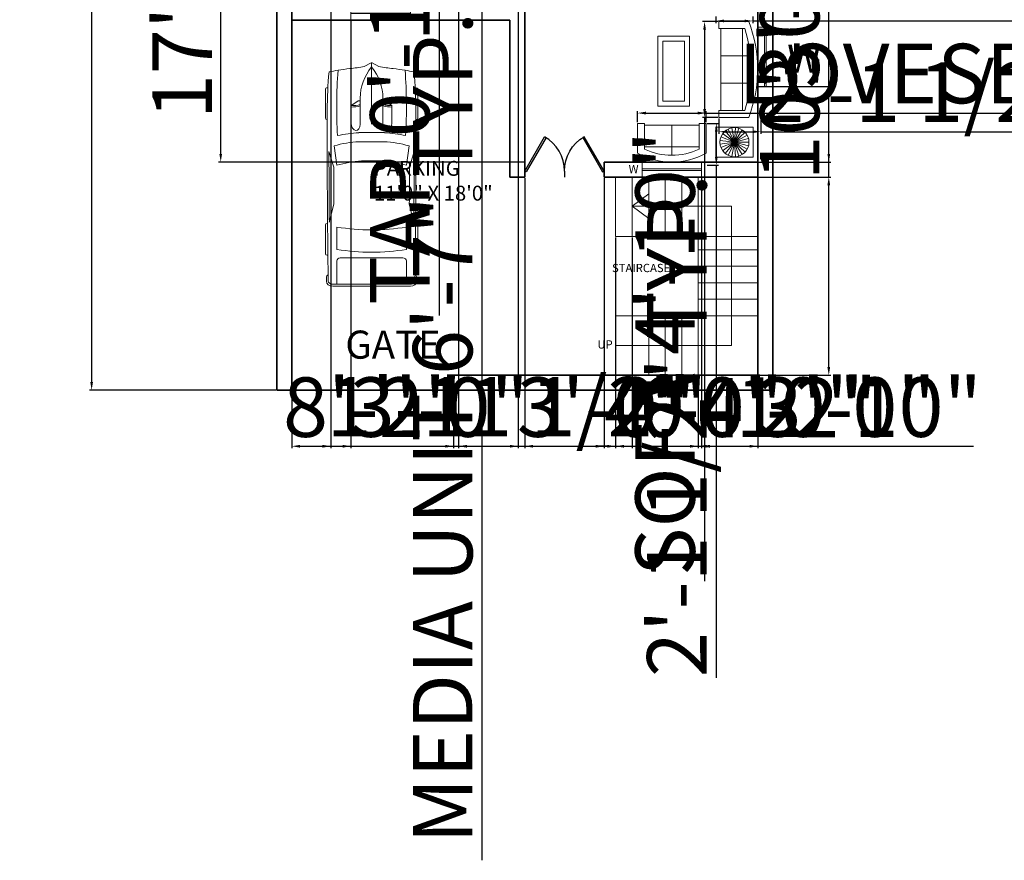
# Model space of a CAD drawing. Units: inches. Extents: x 2901 to 21549, y 2042 to 3828.
# Tile 1 of 10: x 3178 to 3774, y 2590 to 3099. Entities that reach past the tile are written whole.
import ezdxf

# ---------------------------------------------------------------- set-up
doc = ezdxf.new("R2010")
doc.units = ezdxf.units.IN
doc.layers.get('Defpoints').update_dxf_attribs({"color": 1})
for name, color, linetype, lineweight in [('A-ANNO-DIMS', 2, 'Continuous', 18), ('A-ANNO-TEXT', 7, 'Continuous', 18), ('A-AREA-IDEN', 7, 'Continuous', 18), ('A-DOOR', 3, 'Continuous', 25), ('A-FLOR-STRS', 7, 'Continuous', 20), ('A-FURN', 8, 'Continuous', 18), ('A-GLAZ', 4, 'Continuous', 18), ('A-SITE-PARK', 8, 'Continuous', 18), ('A-WALL', 7, 'Continuous', 35)]:
    doc.layers.add(name, color=color, linetype=linetype, lineweight=lineweight)
doc.styles.get("Standard").update_dxf_attribs({"font": 'arial.ttf'})
doc.dimstyles.new('ISO-25', dxfattribs={"dimtxt": 36, "dimasz": 5, "dimexe": 1.25, "dimexo": 0.625, "dimtad": 1, "dimdec": 0, "dimlunit": 3, "dimtxsty": 'Standard', "dimcen": 2.5, "dimadec": 0, "dimazin": 0, "dimtfac": 1, "dimtdec": 0, "dimtmove": 0, "dimatfit": 3, "dimfxl": 1, "dimarcsym": 0})

# ---------------------------------------------------------------- blocks, each defined once
blk = doc.blocks.new('*U23')
for p, q in [((0, 0), (0, -6)), ((40, 0), (40, -6))]:
    blk.add_line(p, q)
blk.add_lwpolyline([(0, 0), (20, 34.64), (21.52, 33.77), (1.52, -0.88)], close=True)
blk.add_arc((0, 0), 40, 0, 60)
blk = doc.blocks.new('Sofa - Roundback 7 ft.')
for p, q in [((-12.00002, -32.4421), (-12.00003, -6.5971)), ((11.99997, -32.4421), (11.99998, -6.5971)), ((-36.000027, -34), (-36.000027, -11.4696)), ((-35.999844, -13.3819), (35.9998, -13.3819)), ((35.99998, -34), (35.99998, -11.4696)), ((-36.000027, -32.4421), (35.99998, -32.4421))]:
    blk.add_line(p, q)
for points in [[(-36.000027, -34), (-42.000027, -34), (-42.000027, -8)], [(41.99998, -8), (41.99998, -34), (35.99998, -34)]]:
    blk.add_lwpolyline(points)
for centre, radius, start, end in [((0, -114.25), 114.25, 68.43141, 111.5686), ((-0.00001, -127.1968), 121.1968, 72.72033, 107.2797)]:
    blk.add_arc(centre, radius, start, end)
blk = doc.blocks.new('Sofa - Roundback Loveseat 5 ft.')
for p, q in [((0, -32.44198), (0, -5.99998)), ((-24, -33.99998), (-24, -11.46958)), ((-23.9998, -13.38178), (23.99986, -13.38178)), ((24.00004, -33.99998), (24.00004, -11.46958)), ((-24, -32.44198), (24.00004, -32.44198))]:
    blk.add_line(p, q)
for points in [[(-24, -33.99998), (-30, -33.99998), (-30, -7.99998)], [(30.00004, -7.99998), (30.00004, -33.99998), (24.00004, -33.99998)]]:
    blk.add_lwpolyline(points)
for centre, radius, start, end in [((0, -60.24998), 60.24998, 60.13715, 119.8628), ((0, -61.38438), 55.38444, 64.32083, 115.6792)]:
    blk.add_arc(centre, radius, start, end)
blk = doc.blocks.new('*U29')
for p, q in [((536, 950), (536, 936)), ((1182, 988), (568, 988)), ((1214, 950), (1214, 950)), ((2235, 810), (1899, 912)), ((3412, 904), (3030, 807)), ((3440, 942), (3440, 950)), ((3472, 988), (4087, 988)), ((4119, 950), (4119, 934)), ((4736, -851), (4736, 851)), ((1779, 801), (2195, 746)), ((3516, 746), (3994, 746)), ((4179, 670), (4179, -670)), ((4736, 746), (4242, 746)), ((4785, -832), (4785, 832)), ((820, 295), (918, 436)), ((918, 436), (1294, 436)), ((756, 241), (1313, 241)), ((816, 241), (816, 283)), ((1496, -274), (1496, 274)), ((1690, -267), (1690, 267)), ((2102, 216), (2102, -216)), ((4736, -267), (4736, 267)), ((83, 156), (3, 10)), ((0, 0), (1313, 0)), ((3, -10), (83, -156)), ((756, -241), (1313, -241)), ((816, -241), (816, -283)), ((820, -295), (918, -436)), ((918, -436), (1294, -436)), ((2195, -746), (1779, -801)), ((2235, -810), (1899, -912)), ((3412, -904), (3030, -807)), ((3994, -746), (3516, -746)), ((4242, -746), (4736, -746)), ((536, -950), (536, -936)), ((1182, -988), (568, -988)), ((1214, -950), (1214, -950)), ((3440, -942), (3440, -950)), ((3472, -988), (4087, -988)), ((4119, -950), (4119, -934))]:
    blk.add_line(p, q)
for centre, major_axis, ratio, start_param, end_param in [((6757, -699), (0, 7958), 0.842304, 1.367076, 1.39176), ((1046, -12468), (0, 13417), 0.842304, 0.00281, 0.075598), ((568, 950), (0, -37.6), 0.842304, 3.141593, 4.712389), ((1638, -268113), (0, 269063), 0.842304, -0.013397, 0.002797), ((1182, 950), (0, 37.6), 0.842304, -1.570796, 0), ((1638, -268113), (0, -269025), 0.842304, 3.133765, 3.140441), ((3472, 950), (0, -37.6), 0.842304, 3.141593, 4.712389), ((4087, 950), (0, 37.6), 0.842304, -1.570796, 0), ((4588, 910), (0, 56.4), 0.842304, -0.013017, 1.249894), ((1638, -268131), (0, 269121), 0.842304, -0.013397, -0.013017), ((4673, 851), (0, -75.2), 0.842304, 1.570796, 3.128196), ((4673, 832), (0, -133), 0.842304, 1.570796, 3.128196), ((6583, -699), (0, -7755), 0.842304, 4.528606, 4.561838), ((952, -15087), (0, -15833), 0.842304, 3.096046, 3.200911), ((3414, 137), (0, -2280), 0.842304, 4.449482, 4.652344), ((3436, 137), (0, 2077), 0.842304, 1.245306, 1.50788), ((3800, 71), (0, -2021), 0.842304, 4.372215, 4.640744), ((2433, -93125), (0, -93935), 0.842304, 3.134049, 3.144098), ((434, 0), (0, 3734), 0.842304, 4.511394, 4.913384), ((912, 0), (0, 3734), 0.842304, 4.511394, 4.913384), ((4242, 670), (0, 75.2), 0.842304, 0, 1.570796), ((-5194, 1331), (0, -6374), 0.842304, 1.385369, 1.434372), ((331, 432), (0, 696), 0.842304, 4.435146, 4.718221), ((361, 432), (0, 696), 0.842304, 4.435146, 4.718221), ((1290, 339), (161, -9), 0.603834, -1.395552, 1.581315), ((756, -1185), (0, 1427), 0.842304, 0, 0.590319), ((832, 283), (0, 18.8), 0.842304, 0.879714, 1.570796), ((16, 0), (0, -18.8), 0.842304, 4.131459, 5.293319), ((-5194, -1331), (0, 6374), 0.842304, -1.434372, -1.385369), ((756, 1185), (0, 1427), 0.842304, 2.551274, 3.141593), ((832, -283), (0, -18.8), 0.842304, 4.712389, 5.403472), ((331, -432), (0, -696), 0.842304, 1.564964, 1.848039), ((361, -432), (0, -696), 0.842304, 1.564964, 1.848039), ((3414, -137), (0, -2280), 0.842304, -1.510751, -1.307889), ((3436, -137), (0, -2077), 0.842304, -1.50788, -1.245306), ((3800, -71), (0, -2021), 0.842304, -1.499151, -1.230623), ((6583, 699), (0, 7755), 0.842304, 1.721348, 1.754579), ((6757, 699), (0, 7958), 0.842304, 1.749832, 1.774517), ((952, 15087), (0, -15833), 0.842304, -0.059319, 0.045547), ((2433, 93125), (0, -93935), 0.842304, -0.002505, 0.007544), ((4242, -670), (0, -75.2), 0.842304, 4.712389, 6.283185), ((4673, -832), (0, -133), 0.842304, 0.013397, 1.570796), ((1046, 12468), (0, -13417), 0.842304, -0.075598, -0.00281), ((568, -950), (0, 37.6), 0.842304, 1.570796, 3.141593), ((1638, 268113), (0, 269063), 0.842304, 3.138796, 3.15499), ((1182, -950), (0, -37.6), 0.842304, 0, 1.570796), ((1638, 268113), (0, -269025), 0.842304, 0.001152, 0.007828), ((3472, -950), (0, -37.6), 0.842304, -1.570796, 0), ((4087, -950), (0, 37.6), 0.842304, 3.141593, 4.712389), ((4588, -910), (0, -56.4), 0.842304, -1.249894, 0.013017), ((1638, 268131), (0, 269121), 0.842304, 3.15461, 3.15499), ((4673, -851), (0, 75.2), 0.842304, 3.15499, 4.712389)]:
    blk.add_ellipse(centre, major_axis=major_axis, ratio=ratio, start_param=start_param, end_param=end_param)
at = {"extrusion": (0, 0, -1)}
blk.add_ellipse((1290, -339), major_axis=(161, 9), ratio=0.603834, start_param=-1.395552, end_param=1.581315, dxfattribs=at)
blk = doc.blocks.new('*D31')
at = {"layer": 'A-ANNO-DIMS', "color": 0, "lineweight": -2, "transparency": 16777216}
for p, q in [((3333.44, 3474.48), (3220.78, 3474.48)), ((3222.03, 3469.48), (3222.03, 2879.48)), ((3333.44, 2874.48), (3220.78, 2874.48))]:
    blk.add_line(p, q, dxfattribs=at)
at = {"layer": 'A-ANNO-DIMS', "color": 0, "transparency": 16777216}
for points in [[(3221.19, 3469.48), (3222.86, 3469.48), (3222.03, 3474.48)], [(3221.19, 2879.48), (3222.86, 2879.48), (3222.03, 2874.48)]]:
    blk.add_solid(points, dxfattribs=at)
at = {"layer": 'Defpoints', "color": 0, "transparency": 16777216}
for p in [(3334.07, 3474.48), (3222.03, 2874.48), (3334.07, 2874.48)]:
    blk.add_point(p, dxfattribs=at)
at = {"layer": 'A-ANNO-DIMS', "color": 0, "transparency": 16777216, "insert": (3203.02, 3174.48), "char_height": 36, "attachment_point": 5, "rotation": 90}
blk.add_mtext("50'", dxfattribs=at)
blk = doc.blocks.new('WIN-36IN-9IN-WALL')
for p, q in [((0, 36), (9, 36)), ((0, 0), (0, 36)), ((4, 0), (4, 36)), ((5, 36), (5, 0)), ((9, 36), (9, 0)), ((9, 0), (0, 0))]:
    blk.add_line(p, q)
blk = doc.blocks.new('*U24')
blk.add_line((-4.41, 0), (4.41, 0))
blk = doc.blocks.new('*U25')
at = {"color": 0, "linetype": 'ByBlock', "lineweight": -2, "transparency": 16777216}
for p, rotation in [((3609.05, 3028.55), 115.1999999999997), ((3610.1, 3028.89), 100.7999999999996), ((3611.21, 3028.96), 86.39999999999972), ((3612.29, 3028.76), 71.99999999999977), ((3606.83, 3026.19), 158.3999999999996), ((3607.36, 3027.15), 143.9999999999996), ((3608.12, 3027.96), 129.5999999999996), ((3613.29, 3028.29), 57.59999999999982), ((3614.14, 3027.58), 43.19999999999986), ((3614.79, 3026.69), 28.7999999999999), ((3615.2, 3025.66), 14.39999999999998), ((3606.56, 3025.12), 172.7999999999996), ((3606.56, 3024.01), 187.1999999999994), ((3606.83, 3022.94), 201.5999999999995), ((3607.36, 3021.97), 215.9999999999995), ((3608.12, 3021.17), 230.3999999999995), ((3609.05, 3020.58), 244.7999999999995), ((3610.1, 3020.23), 259.1999999999994), ((3611.21, 3020.17), 273.5999999999994), ((3612.29, 3020.37), 287.9999999999993), ((3613.29, 3020.84), 302.3999999999992), ((3614.14, 3021.55), 316.7999999999993), ((3614.79, 3022.44), 331.1999999999992), ((3615.2, 3023.47), 345.5999999999992)]:
    blk.add_blockref('*U24', p, dxfattribs=dict(at, rotation=rotation))
blk.add_blockref('*U24', (3615.34, 3024.56), dxfattribs=at)
blk = doc.blocks.new('TABLE-END-DECOR')
blk.add_lwpolyline([(0, 18.24), (22.47, 18.24), (22.47, 0), (0, 0)], close=True)
blk.add_circle((11.23, 9.12), 8.81)
blk.add_blockref('*U25', (-3599.7, -3015.44))
blk = doc.blocks.new('*D44')
at = {"layer": 'A-ANNO-DIMS', "color": 0, "lineweight": -2, "transparency": 16777216}
for p, q in [((3432.19, 3305.97), (3432.19, 3310.97)), ((3431.32, 3300.97), (3433.44, 3300.97)), ((3432.19, 3300.97), (3432.19, 3290.97)), ((3431.32, 3290.97), (3433.44, 3290.97)), ((3432.19, 3285.97), (3432.19, 2919.63))]:
    blk.add_line(p, q, dxfattribs=at)
at = {"layer": 'A-ANNO-DIMS', "color": 0, "transparency": 16777216}
for points in [[(3431.36, 3305.97), (3433.02, 3305.97), (3432.19, 3300.97)], [(3431.36, 3285.97), (3433.02, 3285.97), (3432.19, 3290.97)]]:
    blk.add_solid(points, dxfattribs=at)
at = {"layer": 'Defpoints', "color": 0, "transparency": 16777216}
for p in [(3430.69, 3300.97), (3430.69, 3290.97), (3432.19, 3290.97)]:
    blk.add_point(p, dxfattribs=at)
at = {"layer": 'A-ANNO-DIMS', "color": 0, "transparency": 16777216, "insert": (3413.18, 3100.3), "char_height": 36, "attachment_point": 5, "rotation": 90}
blk.add_mtext('TAP 0\'-10" TYP.', dxfattribs=at)
blk = doc.blocks.new('*D48')
at = {"layer": 'A-ANNO-DIMS', "color": 0, "lineweight": -2, "transparency": 16777216}
for p, q in [((3552.33, 3036.58), (3552.33, 3043.43)), ((3557.33, 3042.18), (3588.77, 3042.18)), ((3593.77, 3036.58), (3593.77, 3043.43)), ((3593.77, 3042.18), (4181.25, 3042.18))]:
    blk.add_line(p, q, dxfattribs=at)
at = {"layer": 'A-ANNO-DIMS', "color": 0, "transparency": 16777216}
for points in [[(3557.33, 3043.01), (3557.33, 3041.34), (3552.33, 3042.18)], [(3588.77, 3043.01), (3588.77, 3041.34), (3593.77, 3042.18)]]:
    blk.add_solid(points, dxfattribs=at)
at = {"layer": 'Defpoints', "color": 0, "transparency": 16777216}
for p in [(3593.77, 3042.18), (3552.33, 3035.96), (3593.77, 3035.96)]:
    blk.add_point(p, dxfattribs=at)
at = {"layer": 'A-ANNO-DIMS', "color": 0, "transparency": 16777216, "insert": (3890.01, 3061.44), "char_height": 36, "attachment_point": 5}
blk.add_mtext('LOVESEAT 3\'-5 1/2" TYP.', dxfattribs=at)
blk = doc.blocks.new('*D49')
at = {"layer": 'A-ANNO-DIMS', "color": 0, "lineweight": -2, "transparency": 16777216}
for p, q in [((3594.39, 3035.96), (3601.23, 3035.96)), ((3599.98, 3030.96), (3599.98, 3015.64)), ((3594.39, 3010.64), (3601.23, 3010.64)), ((3599.98, 3010.64), (3599.98, 2700.45))]:
    blk.add_line(p, q, dxfattribs=at)
at = {"layer": 'A-ANNO-DIMS', "color": 0, "transparency": 16777216}
for points in [[(3599.15, 3030.96), (3600.81, 3030.96), (3599.98, 3035.96)], [(3599.15, 3015.64), (3600.81, 3015.64), (3599.98, 3010.64)]]:
    blk.add_solid(points, dxfattribs=at)
at = {"layer": 'Defpoints', "color": 0, "transparency": 16777216}
for p in [(3593.77, 3035.96), (3593.77, 3010.64), (3599.98, 3010.64)]:
    blk.add_point(p, dxfattribs=at)
at = {"layer": 'A-ANNO-DIMS', "color": 0, "transparency": 16777216, "insert": (3580.74, 2853.04), "char_height": 36, "attachment_point": 5, "rotation": 90}
blk.add_mtext('2\'-1 1/2" TYP.', dxfattribs=at)
blk = doc.blocks.new('*D50')
at = {"layer": 'A-ANNO-DIMS', "color": 0, "lineweight": -2, "transparency": 16777216}
for p, q in [((3599.61, 3100.68), (3599.61, 3096.69)), ((3604.61, 3097.94), (3617.08, 3097.94)), ((3622.08, 3100.68), (3622.08, 3096.69)), ((3622.08, 3097.94), (4251.18, 3097.94))]:
    blk.add_line(p, q, dxfattribs=at)
at = {"layer": 'A-ANNO-DIMS', "color": 0, "transparency": 16777216}
for points in [[(3604.61, 3098.77), (3604.61, 3097.1), (3599.61, 3097.94)], [(3617.08, 3098.77), (3617.08, 3097.1), (3622.08, 3097.94)]]:
    blk.add_solid(points, dxfattribs=at)
at = {"layer": 'Defpoints', "color": 0, "transparency": 16777216}
for p in [(3599.61, 3101.31), (3622.08, 3101.31), (3622.08, 3097.94)]:
    blk.add_point(p, dxfattribs=at)
at = {"layer": 'A-ANNO-DIMS', "color": 0, "transparency": 16777216, "insert": (3939.13, 3117.18), "char_height": 36, "attachment_point": 5}
blk.add_mtext('END TABLE 1\'-10 1/2" TYP.', dxfattribs=at)
blk = doc.blocks.new('*D52')
at = {"layer": 'A-ANNO-DIMS', "color": 0, "lineweight": -2, "transparency": 16777216}
for p, q in [((3469.26, 3197.35), (3456.81, 3197.35)), ((3458.06, 3192.35), (3458.06, 3123.52)), ((3469.26, 3118.52), (3456.81, 3118.52)), ((3458.06, 3118.52), (3458.06, 2589.92))]:
    blk.add_line(p, q, dxfattribs=at)
at = {"layer": 'A-ANNO-DIMS', "color": 0, "transparency": 16777216}
for points in [[(3457.23, 3192.35), (3458.9, 3192.35), (3458.06, 3197.35)], [(3457.23, 3123.52), (3458.9, 3123.52), (3458.06, 3118.52)]]:
    blk.add_solid(points, dxfattribs=at)
at = {"layer": 'Defpoints', "color": 0, "transparency": 16777216}
for p in [(3469.89, 3197.35), (3458.06, 3118.52), (3469.89, 3118.52)]:
    blk.add_point(p, dxfattribs=at)
at = {"layer": 'A-ANNO-DIMS', "color": 0, "transparency": 16777216, "insert": (3439.06, 2851.72), "char_height": 36, "attachment_point": 5, "rotation": 90}
blk.add_mtext('MEDIA UNIT 6\'-7" TYP.', dxfattribs=at)
blk = doc.blocks.new('*D54')
at = {"layer": 'A-ANNO-DIMS', "color": 0, "lineweight": -2, "transparency": 16777216}
for p, q in [((3536.12, 3164.87), (3536.12, 3153.97)), ((3604.61, 3164.87), (3604.61, 3153.97)), ((3541.12, 3155.22), (3599.61, 3155.22)), ((3604.61, 3155.22), (4090.43, 3155.22))]:
    blk.add_line(p, q, dxfattribs=at)
at = {"layer": 'A-ANNO-DIMS', "color": 0, "transparency": 16777216}
for points in [[(3541.12, 3156.05), (3541.12, 3154.38), (3536.12, 3155.22)], [(3599.61, 3156.05), (3599.61, 3154.38), (3604.61, 3155.22)]]:
    blk.add_solid(points, dxfattribs=at)
at = {"layer": 'Defpoints', "color": 0, "transparency": 16777216}
for p in [(3536.12, 3165.49), (3604.61, 3165.49), (3604.61, 3155.22)]:
    blk.add_point(p, dxfattribs=at)
at = {"layer": 'A-ANNO-DIMS', "color": 0, "transparency": 16777216, "insert": (3850.02, 3174.46), "char_height": 36, "attachment_point": 5}
blk.add_mtext('DINING SET 5\'-8 1/2"', dxfattribs=at)
blk = doc.blocks.new('*D56')
at = {"layer": 'A-ANNO-DIMS', "color": 0, "lineweight": -2, "transparency": 16777216}
for p, q in [((3600.96, 3097.61), (3591.63, 3097.61)), ((3592.88, 3092.61), (3592.88, 3044.6)), ((3600.96, 3039.6), (3591.63, 3039.6)), ((3592.88, 3039.6), (3592.88, 2758.95))]:
    blk.add_line(p, q, dxfattribs=at)
at = {"layer": 'A-ANNO-DIMS', "color": 0, "transparency": 16777216}
for points in [[(3592.05, 3092.61), (3593.72, 3092.61), (3592.88, 3097.61)], [(3592.05, 3044.6), (3593.72, 3044.6), (3592.88, 3039.6)]]:
    blk.add_solid(points, dxfattribs=at)
at = {"layer": 'Defpoints', "color": 0, "transparency": 16777216}
for p in [(3601.59, 3097.61), (3592.88, 3039.6), (3601.59, 3039.6)]:
    blk.add_point(p, dxfattribs=at)
at = {"layer": 'A-ANNO-DIMS', "color": 0, "transparency": 16777216, "insert": (3573.63, 2896.77), "char_height": 36, "attachment_point": 5, "rotation": 90}
blk.add_mtext('SOFA 4\'-10"', dxfattribs=at)
blk = doc.blocks.new('*D57')
at = {"layer": 'A-ANNO-DIMS', "color": 0, "lineweight": -2, "transparency": 16777216}
for p, q in [((3601.59, 3038.97), (3601.59, 3029.64)), ((3626.91, 3038.97), (3626.91, 3029.64)), ((3606.59, 3030.89), (3621.91, 3030.89)), ((3626.91, 3030.89), (3813.36, 3030.89))]:
    blk.add_line(p, q, dxfattribs=at)
at = {"layer": 'A-ANNO-DIMS', "color": 0, "transparency": 16777216}
for points in [[(3606.59, 3031.73), (3606.59, 3030.06), (3601.59, 3030.89)], [(3621.91, 3031.73), (3621.91, 3030.06), (3626.91, 3030.89)]]:
    blk.add_solid(points, dxfattribs=at)
at = {"layer": 'Defpoints', "color": 0, "transparency": 16777216}
for p in [(3601.59, 3039.6), (3626.91, 3039.6), (3626.91, 3030.89)]:
    blk.add_point(p, dxfattribs=at)
at = {"layer": 'A-ANNO-DIMS', "color": 0, "transparency": 16777216, "insert": (3722.63, 3050.13), "char_height": 36, "attachment_point": 5}
blk.add_mtext('2\'-1 1/2"', dxfattribs=at)
blk = doc.blocks.new('*D62')
at = {"layer": 'A-ANNO-DIMS', "color": 0, "lineweight": -2, "transparency": 16777216}
for p, q in [((3343.07, 2873.85), (3343.07, 2839.28)), ((3441, 2873.85), (3441, 2839.28)), ((3348.07, 2840.53), (3436, 2840.53))]:
    blk.add_line(p, q, dxfattribs=at)
at = {"layer": 'A-ANNO-DIMS', "color": 0, "transparency": 16777216}
for points in [[(3348.07, 2841.36), (3348.07, 2839.69), (3343.07, 2840.53)], [(3436, 2841.36), (3436, 2839.69), (3441, 2840.53)]]:
    blk.add_solid(points, dxfattribs=at)
at = {"layer": 'Defpoints', "color": 0, "transparency": 16777216}
for p in [(3343.07, 2874.48), (3441, 2874.48), (3441, 2840.53)]:
    blk.add_point(p, dxfattribs=at)
at = {"layer": 'A-ANNO-DIMS', "color": 0, "transparency": 16777216, "insert": (3392.04, 2859.53), "char_height": 36, "attachment_point": 5}
blk.add_mtext('8\'-2"', dxfattribs=at)
blk = doc.blocks.new('*D63')
at = {"layer": 'A-ANNO-DIMS', "color": 0, "lineweight": -2, "transparency": 16777216}
for p, q in [((3539.07, 2882.85), (3539.07, 2839.28)), ((3589.07, 2882.85), (3589.07, 2839.28)), ((3544.07, 2840.53), (3584.07, 2840.53)), ((3589.07, 2840.53), (3692.47, 2840.53))]:
    blk.add_line(p, q, dxfattribs=at)
at = {"layer": 'A-ANNO-DIMS', "color": 0, "transparency": 16777216}
for points in [[(3544.07, 2841.36), (3544.07, 2839.69), (3539.07, 2840.53)], [(3584.07, 2841.36), (3584.07, 2839.69), (3589.07, 2840.53)]]:
    blk.add_solid(points, dxfattribs=at)
at = {"layer": 'Defpoints', "color": 0, "transparency": 16777216}
for p in [(3539.07, 2883.48), (3589.07, 2883.48), (3589.07, 2840.53)]:
    blk.add_point(p, dxfattribs=at)
at = {"layer": 'A-ANNO-DIMS', "color": 0, "transparency": 16777216, "insert": (3643.27, 2859.23), "char_height": 36, "attachment_point": 5}
blk.add_mtext('4\'-2"', dxfattribs=at)
blk = doc.blocks.new('*D64')
at = {"layer": 'A-ANNO-DIMS', "color": 0, "lineweight": -2, "transparency": 16777216}
for p, q in [((3589.07, 2882.85), (3589.07, 2839.28)), ((3625.07, 2882.85), (3625.07, 2839.28)), ((3594.07, 2840.53), (3620.07, 2840.53)), ((3625.07, 2840.53), (3726.99, 2840.53))]:
    blk.add_line(p, q, dxfattribs=at)
at = {"layer": 'A-ANNO-DIMS', "color": 0, "transparency": 16777216}
for points in [[(3594.07, 2841.36), (3594.07, 2839.69), (3589.07, 2840.53)], [(3620.07, 2841.36), (3620.07, 2839.69), (3625.07, 2840.53)]]:
    blk.add_solid(points, dxfattribs=at)
at = {"layer": 'Defpoints', "color": 0, "transparency": 16777216}
for p in [(3589.07, 2883.48), (3625.07, 2883.48), (3625.07, 2840.53)]:
    blk.add_point(p, dxfattribs=at)
at = {"layer": 'A-ANNO-DIMS', "color": 0, "transparency": 16777216, "insert": (3678.53, 2859.55), "char_height": 36, "attachment_point": 5}
blk.add_mtext('3\'-0"', dxfattribs=at)
blk = doc.blocks.new('*D65')
at = {"layer": 'A-ANNO-DIMS', "color": 0, "lineweight": -2, "transparency": 16777216}
for p, q in [((3668.02, 3003.48), (3668.02, 3130.01)), ((3625.69, 3003.48), (3669.27, 3003.48)), ((3668.02, 2888.48), (3668.02, 2998.48)), ((3625.69, 2883.48), (3669.27, 2883.48))]:
    blk.add_line(p, q, dxfattribs=at)
at = {"layer": 'A-ANNO-DIMS', "color": 0, "transparency": 16777216}
for points in [[(3667.19, 2998.48), (3668.85, 2998.48), (3668.02, 3003.48)], [(3667.19, 2888.48), (3668.85, 2888.48), (3668.02, 2883.48)]]:
    blk.add_solid(points, dxfattribs=at)
at = {"layer": 'Defpoints', "color": 0, "transparency": 16777216}
for p in [(3625.07, 3003.48), (3668.02, 3003.48), (3625.07, 2883.48)]:
    blk.add_point(p, dxfattribs=at)
at = {"layer": 'A-ANNO-DIMS', "color": 0, "transparency": 16777216, "insert": (3649.01, 3069.24), "char_height": 36, "attachment_point": 5, "rotation": 90}
blk.add_mtext('10\'-0"', dxfattribs=at)
blk = doc.blocks.new('*D66')
at = {"layer": 'A-ANNO-DIMS', "color": 0, "lineweight": -2, "transparency": 16777216}
for p, q in [((3484.07, 3002.85), (3484.07, 2839.28)), ((3532.07, 3002.85), (3532.07, 2839.28)), ((3489.07, 2840.53), (3527.07, 2840.53)), ((3532.07, 2840.53), (3635.47, 2840.53))]:
    blk.add_line(p, q, dxfattribs=at)
at = {"layer": 'A-ANNO-DIMS', "color": 0, "transparency": 16777216}
for points in [[(3489.07, 2841.36), (3489.07, 2839.69), (3484.07, 2840.53)], [(3527.07, 2841.36), (3527.07, 2839.69), (3532.07, 2840.53)]]:
    blk.add_solid(points, dxfattribs=at)
at = {"layer": 'Defpoints', "color": 0, "transparency": 16777216}
for p in [(3484.07, 3003.48), (3532.07, 3003.48), (3532.07, 2840.53)]:
    blk.add_point(p, dxfattribs=at)
at = {"layer": 'A-ANNO-DIMS', "color": 0, "transparency": 16777216, "insert": (3586.27, 2859.53), "char_height": 36, "attachment_point": 5}
blk.add_mtext('4\'-0"', dxfattribs=at)
blk = doc.blocks.new('*D67')
at = {"layer": 'A-ANNO-DIMS', "color": 0, "lineweight": -2, "transparency": 16777216}
for p, q in [((3484.07, 3013.1), (3484.07, 3509.68)), ((3625.07, 3228.1), (3625.07, 3509.68)), ((3489.07, 3508.43), (3620.07, 3508.43))]:
    blk.add_line(p, q, dxfattribs=at)
at = {"layer": 'A-ANNO-DIMS', "color": 0, "transparency": 16777216}
for points in [[(3489.07, 3509.26), (3489.07, 3507.59), (3484.07, 3508.43)], [(3620.07, 3509.26), (3620.07, 3507.59), (3625.07, 3508.43)]]:
    blk.add_solid(points, dxfattribs=at)
at = {"layer": 'Defpoints', "color": 0, "transparency": 16777216}
for p in [(3625.07, 3508.43), (3625.07, 3227.48), (3484.07, 3012.48)]:
    blk.add_point(p, dxfattribs=at)
at = {"layer": 'A-ANNO-DIMS', "color": 0, "transparency": 16777216, "insert": (3554.57, 3527.43), "char_height": 36, "attachment_point": 5}
blk.add_mtext('11\'-9"', dxfattribs=at)
blk = doc.blocks.new('*D68')
at = {"layer": 'A-ANNO-DIMS', "color": 0, "lineweight": -2, "transparency": 16777216}
for p, q in [((3531.44, 3227.48), (3298.87, 3227.48)), ((3300.12, 3017.48), (3300.12, 3222.48)), ((3483.44, 3012.48), (3298.87, 3012.48))]:
    blk.add_line(p, q, dxfattribs=at)
at = {"layer": 'A-ANNO-DIMS', "color": 0, "transparency": 16777216}
for points in [[(3299.29, 3222.48), (3300.95, 3222.48), (3300.12, 3227.48)], [(3299.29, 3017.48), (3300.95, 3017.48), (3300.12, 3012.48)]]:
    blk.add_solid(points, dxfattribs=at)
at = {"layer": 'Defpoints', "color": 0, "transparency": 16777216}
for p in [(3300.12, 3227.48), (3532.07, 3227.48), (3484.07, 3012.48)]:
    blk.add_point(p, dxfattribs=at)
at = {"layer": 'A-ANNO-DIMS', "color": 0, "transparency": 16777216, "insert": (3281.42, 3119.98), "char_height": 36, "attachment_point": 5, "rotation": 90}
blk.add_mtext('17\'-11"', dxfattribs=at)
blk = doc.blocks.new('*D73')
at = {"layer": 'A-ANNO-DIMS', "color": 0, "lineweight": -2, "transparency": 16777216}
for p, q in [((3668.02, 3058.19), (3668.02, 3244)), ((3625.69, 3058.19), (3669.27, 3058.19)), ((3668.02, 3017.48), (3668.02, 3053.19)), ((3625.69, 3012.48), (3669.27, 3012.48))]:
    blk.add_line(p, q, dxfattribs=at)
at = {"layer": 'A-ANNO-DIMS', "color": 0, "transparency": 16777216}
for points in [[(3667.19, 3053.19), (3668.85, 3053.19), (3668.02, 3058.19)], [(3667.19, 3017.48), (3668.85, 3017.48), (3668.02, 3012.48)]]:
    blk.add_solid(points, dxfattribs=at)
at = {"layer": 'Defpoints', "color": 0, "transparency": 16777216}
for p in [(3625.07, 3058.19), (3668.02, 3058.19), (3625.07, 3012.48)]:
    blk.add_point(p, dxfattribs=at)
at = {"layer": 'A-ANNO-DIMS', "color": 0, "transparency": 16777216, "insert": (3648.77, 3153.6), "char_height": 36, "attachment_point": 5, "rotation": 90}
blk.add_mtext('3\'-9 1/2"', dxfattribs=at)
blk = doc.blocks.new('*D75')
at = {"layer": 'A-ANNO-DIMS', "color": 0, "lineweight": -2, "transparency": 16777216}
for p, q in [((3343.07, 3097.85), (3343.07, 2839.28)), ((3378.91, 3097.85), (3378.91, 2839.28)), ((3348.07, 2840.53), (3373.91, 2840.53)), ((3378.91, 2840.53), (3480.83, 2840.53))]:
    blk.add_line(p, q, dxfattribs=at)
at = {"layer": 'A-ANNO-DIMS', "color": 0, "transparency": 16777216}
for points in [[(3348.07, 2841.36), (3348.07, 2839.69), (3343.07, 2840.53)], [(3373.91, 2841.36), (3373.91, 2839.69), (3378.91, 2840.53)]]:
    blk.add_solid(points, dxfattribs=at)
at = {"layer": 'Defpoints', "color": 0, "transparency": 16777216}
for p in [(3343.07, 3098.48), (3378.91, 3098.48), (3378.91, 2840.53)]:
    blk.add_point(p, dxfattribs=at)
at = {"layer": 'A-ANNO-DIMS', "color": 0, "transparency": 16777216, "insert": (3432.37, 2859.55), "char_height": 36, "attachment_point": 5}
blk.add_mtext('3\'-0"', dxfattribs=at)
blk = doc.blocks.new('*D76')
at = {"layer": 'A-ANNO-DIMS', "color": 0, "lineweight": -2, "transparency": 16777216}
for p, q in [((3591.05, 3002.85), (3591.05, 2839.28)), ((3625.07, 3002.85), (3625.07, 2839.28)), ((3596.05, 2840.53), (3620.07, 2840.53)), ((3625.07, 2840.53), (3755.6, 2840.53))]:
    blk.add_line(p, q, dxfattribs=at)
at = {"layer": 'A-ANNO-DIMS', "color": 0, "transparency": 16777216}
for points in [[(3596.05, 2841.36), (3596.05, 2839.69), (3591.05, 2840.53)], [(3620.07, 2841.36), (3620.07, 2839.69), (3625.07, 2840.53)]]:
    blk.add_solid(points, dxfattribs=at)
at = {"layer": 'Defpoints', "color": 0, "transparency": 16777216}
for p in [(3591.05, 3003.48), (3625.07, 3003.48), (3625.07, 2840.53)]:
    blk.add_point(p, dxfattribs=at)
at = {"layer": 'A-ANNO-DIMS', "color": 0, "transparency": 16777216, "insert": (3692.84, 2859.53), "char_height": 36, "attachment_point": 5}
blk.add_mtext('2\'-10"', dxfattribs=at)
blk = doc.blocks.new('*D78')
at = {"layer": 'A-ANNO-DIMS', "color": 0, "lineweight": -2, "transparency": 16777216}
for p, q in [((3343.07, 3230.85), (3343.07, 2839.28)), ((3366.66, 3230.85), (3366.66, 2839.28)), ((3348.07, 2840.53), (3361.66, 2840.53)), ((3366.66, 2840.53), (3577.07, 2840.53))]:
    blk.add_line(p, q, dxfattribs=at)
at = {"layer": 'A-ANNO-DIMS', "color": 0, "transparency": 16777216}
for points in [[(3348.07, 2841.36), (3348.07, 2839.69), (3343.07, 2840.53)], [(3361.66, 2841.36), (3361.66, 2839.69), (3366.66, 2840.53)]]:
    blk.add_solid(points, dxfattribs=at)
at = {"layer": 'Defpoints', "color": 0, "transparency": 16777216}
for p in [(3343.07, 3231.48), (3366.66, 3231.48), (3366.66, 2840.53)]:
    blk.add_point(p, dxfattribs=at)
at = {"layer": 'A-ANNO-DIMS', "color": 0, "transparency": 16777216, "insert": (3474.37, 2859.77), "char_height": 36, "attachment_point": 5}
blk.add_mtext('1\'-11 1/2"', dxfattribs=at)
blk = doc.blocks.new('*D84')
at = {"layer": 'A-ANNO-DIMS', "color": 0, "lineweight": -2, "transparency": 16777216}
for p, q in [((3444.07, 3230.85), (3444.07, 2839.28)), ((3480.07, 3230.85), (3480.07, 2839.28)), ((3449.07, 2840.53), (3475.07, 2840.53)), ((3480.07, 2840.53), (3581.99, 2840.53))]:
    blk.add_line(p, q, dxfattribs=at)
at = {"layer": 'A-ANNO-DIMS', "color": 0, "transparency": 16777216}
for points in [[(3449.07, 2841.36), (3449.07, 2839.69), (3444.07, 2840.53)], [(3475.07, 2841.36), (3475.07, 2839.69), (3480.07, 2840.53)]]:
    blk.add_solid(points, dxfattribs=at)
at = {"layer": 'Defpoints', "color": 0, "transparency": 16777216}
for p in [(3444.07, 3231.48), (3480.07, 3231.48), (3480.07, 2840.53)]:
    blk.add_point(p, dxfattribs=at)
at = {"layer": 'A-ANNO-DIMS', "color": 0, "transparency": 16777216, "insert": (3533.53, 2859.55), "char_height": 36, "attachment_point": 5}
blk.add_mtext('3\'-0"', dxfattribs=at)
blk = doc.blocks.new('*D85')
at = {"layer": 'A-ANNO-DIMS', "color": 0, "lineweight": -2, "transparency": 16777216}
for p, q in [((3539.07, 2966.85), (3539.07, 2839.28)), ((3549.07, 2966.85), (3549.07, 2839.28)), ((3534.07, 2840.53), (3529.07, 2840.53)), ((3539.07, 2840.53), (3549.07, 2840.53)), ((3554.07, 2840.53), (3683.99, 2840.53))]:
    blk.add_line(p, q, dxfattribs=at)
at = {"layer": 'A-ANNO-DIMS', "color": 0, "transparency": 16777216}
for points in [[(3534.07, 2841.36), (3534.07, 2839.69), (3539.07, 2840.53)], [(3554.07, 2841.36), (3554.07, 2839.69), (3549.07, 2840.53)]]:
    blk.add_solid(points, dxfattribs=at)
at = {"layer": 'Defpoints', "color": 0, "transparency": 16777216}
for p in [(3539.07, 2967.48), (3549.07, 2967.48), (3549.07, 2840.53)]:
    blk.add_point(p, dxfattribs=at)
at = {"layer": 'A-ANNO-DIMS', "color": 0, "transparency": 16777216, "insert": (3621.53, 2859.53), "char_height": 36, "attachment_point": 5}
blk.add_mtext('0\'-10"', dxfattribs=at)

msp = doc.modelspace()

# ---------------------------------------------------------------- linework, layer by layer
at = {"layer": 'A-FLOR-STRS'}
for p, q in [((3539.07, 2967.48), (3539.07, 3003.48)), ((3549.07, 2967.48), (3549.07, 3003.48)), ((3559.07, 2967.48), (3559.07, 3003.48)), ((3569.07, 2967.48), (3569.07, 3003.48)), ((3579.07, 2967.48), (3579.07, 3003.48)), ((3589.07, 3003.48), (3589.07, 2967.48)), ((3589.07, 2967.48), (3589.07, 3003.48)), ((3549.07, 2985.89), (3559.07, 2993.4)), ((3609.23, 2985.89), (3549.07, 2985.89)), ((3549.07, 2985.89), (3559.07, 2978.37)), ((3609.23, 2901.48), (3609.23, 2985.89)), ((3625.07, 2967.48), (3539.07, 2967.48)), ((3589.07, 2919.48), (3589.07, 2967.48)), ((3589.07, 2959.48), (3625.07, 2959.48)), ((3589.07, 2949.48), (3625.07, 2949.48)), ((3589.07, 2939.48), (3625.07, 2939.48)), ((3589.07, 2929.48), (3625.07, 2929.48)), ((3625.07, 2919.48), (3539.07, 2919.48)), ((3539.07, 2919.48), (3539.07, 2883.48)), ((3549.07, 2919.48), (3549.07, 2883.48)), ((3559.07, 2919.48), (3559.07, 2883.48)), ((3569.07, 2919.48), (3569.07, 2883.48)), ((3579.07, 2919.48), (3579.07, 2883.48)), ((3589.07, 2919.48), (3589.07, 2883.48)), ((3589.07, 2919.48), (3625.07, 2919.48)), ((3539.07, 2901.48), (3609.23, 2901.48))]:
    msp.add_line(p, q, dxfattribs=at)
at = {"layer": 'A-FURN'}
for points in [[(3564.66, 3088.7), (3583.75, 3088.7), (3583.75, 3046.38), (3564.66, 3046.38)], [(3567.66, 3085.7), (3580.75, 3085.7), (3580.75, 3049.38), (3567.66, 3049.38)]]:
    msp.add_lwpolyline(points, close=True, dxfattribs=at)
at = {"layer": 'A-WALL'}
for p, q in [((3343.07, 2883.48), (3343.07, 3465.48)), ((3625.07, 3465.48), (3625.07, 2883.48)), ((3484.07, 3012.48), (3484.07, 3231.48)), ((3343.07, 3098.48), (3475.07, 3098.48)), ((3475.07, 3003.48), (3475.07, 3098.48)), ((3484.07, 3012.48), (3484.07, 3003.48)), ((3625.07, 3012.48), (3532.07, 3012.48)), ((3532.07, 3012.48), (3532.07, 3003.48)), ((3484.07, 3003.48), (3475.07, 3003.48)), ((3625.07, 3003.48), (3532.07, 3003.48)), ((3343.07, 2883.48), (3343.07, 2874.48)), ((3625.07, 2883.48), (3441, 2883.48)), ((3441, 2874.48), (3441, 2883.48))]:
    msp.add_line(p, q, dxfattribs=at)
msp.add_lwpolyline([(3634.07, 3474.48), (3634.07, 2874.48), (3334.07, 2874.48), (3334.07, 3474.48)], close=True, dxfattribs=at)

# ---------------------------------------------------------------- block references
at = {"layer": 'A-DOOR', "yscale": 0.6000000000000111, "zscale": 0.6000000000000111}
for p, xscale in [((3484.07, 3007.08), 0.6000000000000111), ((3532.07, 3007.08), -0.6000000000000111)]:
    msp.add_blockref('*U23', p, dxfattribs=dict(at, xscale=xscale))
at = {"layer": 'A-FURN', "yscale": 0.690663340395338, "zscale": 0.690663340395338}
for name, p, xscale, rotation in [('Sofa - Roundback 7 ft.', (3625.07, 3068.6), 0.690663340395338, 270), ('Sofa - Roundback Loveseat 5 ft.', (3573.05, 3012.48), -0.690663340395338, 180)]:
    msp.add_blockref(name, p, dxfattribs=dict(at, xscale=xscale, rotation=rotation))
at = {"layer": 'A-FURN'}
msp.add_blockref('TABLE-END-DECOR', (3599.7, 3015.44), dxfattribs=at)
at = {"layer": 'A-GLAZ', "rotation": 270}
for p in [(3378.91, 3107.48), (3555.05, 3012.48)]:
    msp.add_blockref('WIN-36IN-9IN-WALL', p, dxfattribs=at)
at = {"layer": 'A-GLAZ'}
msp.add_blockref('WIN-36IN-9IN-WALL', (3625.07, 3058.19), dxfattribs=at)
at = {"layer": 'A-SITE-PARK', "xscale": 0.0282735901811254, "yscale": 0.0282735901811254, "zscale": 0.0282735901811254, "rotation": 270}
msp.add_blockref('*U29', (3391.39, 3072.63), dxfattribs=at)

# ---------------------------------------------------------------- texts
at = {"layer": 'A-ANNO-TEXT', "attachment_point": 1}
for s, insert, char_height in [('{\\fArial|b1|i0|c0|p34;W}', (3642.89, 3083.54), 17), ('{\\fArial|b1|i0|c0|p34;W}', (3546.92, 3010.79), 5), ('{\\fArial|b1|i0|c0|p34;GATE}', (3375.52, 2910.53), 17), ('{\\fArial|b1|i0|c0|p34;UP}', (3528.03, 2904.65), 5)]:
    msp.add_mtext_dynamic_manual_height_columns(s, width=86.7973, gutter_width=12.5, heights=[27.4], dxfattribs=dict(at, insert=insert, char_height=char_height))
at = {"layer": 'A-AREA-IDEN', "attachment_point": 1}
for s, insert, char_height in [('{\\fArial|b1|i0|c0|p34;PARKING\\P11\'0" X 18\'0"}', (3392.8, 3013.21), 9), ('{\\fArial|b1|i0|c0|p34;STAIRCASE}', (3536.88, 2950.93), 5)]:
    msp.add_mtext_dynamic_manual_height_columns(s, width=86.7973, gutter_width=12.5, heights=[27.4], dxfattribs=dict(at, insert=insert, char_height=char_height))

# ---------------------------------------------------------------- dimensions: what is measured, and where the dimension line sits
at = {"layer": 'A-ANNO-DIMS'}
for base, p1, p2, picture, middle in [((3625.07, 3508.43), (3484.07, 3012.48), (3625.07, 3227.48), '*D67', (3554.57, 3527.43)), ((3366.66, 2840.53), (3343.07, 3231.48), (3366.66, 3231.48), '*D78', (3474.37, 2859.77)), ((3480.07, 2840.53), (3444.07, 3231.48), (3480.07, 3231.48), '*D84', (3533.53, 2859.55)), ((3626.91, 3030.89), (3601.59, 3039.6), (3626.91, 3039.6), '*D57', (3722.63, 3050.13)), ((3378.91, 2840.53), (3343.07, 3098.48), (3378.91, 3098.48), '*D75', (3432.37, 2859.55)), ((3532.07, 2840.53), (3484.07, 3003.48), (3532.07, 3003.48), '*D66', (3586.27, 2859.53)), ((3625.07, 2840.53), (3591.05, 3003.48), (3625.07, 3003.48), '*D76', (3692.84, 2859.53)), ((3549.07, 2840.53), (3539.07, 2967.48), (3549.07, 2967.48), '*D85', (3621.53, 2859.53)), ((3441, 2840.53), (3343.07, 2874.48), (3441, 2874.48), '*D62', (3392.04, 2859.53)), ((3589.07, 2840.53), (3539.07, 2883.48), (3589.07, 2883.48), '*D63', (3643.27, 2859.23)), ((3625.07, 2840.53), (3589.07, 2883.48), (3625.07, 2883.48), '*D64', (3678.53, 2859.55))]:
    dim = msp.add_linear_dim(base=base, p1=p1, p2=p2, dimstyle='ISO-25', override={"dimdec": 1, "dimlfac": 1, "dimrnd": 0, "dimzin": 1, "dimdsep": 46, "dimlunit": 4, "dimfrac": 2}, dxfattribs=at)
    dim.commit()
    dim.dimension.update_dxf_attribs({"geometry": picture, "text_midpoint": middle})
for base, p1, p2, override, picture, middle in [((3222.03, 2874.48), (3334.07, 3474.48), (3334.07, 2874.48), {"dimclrd": 0, "dimclre": 0, "dimclrt": 0}, '*D31', (3203.02, 3174.48)), ((3668.02, 3058.19), (3625.07, 3012.48), (3625.07, 3058.19), {"dimdec": 1, "dimlfac": 1, "dimrnd": 0, "dimzin": 1, "dimdsep": 46, "dimlunit": 4, "dimfrac": 2}, '*D73', (3648.77, 3153.6)), ((3300.12, 3227.48), (3484.07, 3012.48), (3532.07, 3227.48), {"dimdec": 1, "dimlfac": 1, "dimrnd": 0, "dimzin": 1, "dimdsep": 46, "dimlunit": 4, "dimfrac": 2}, '*D68', (3281.42, 3119.98)), ((3668.02, 3003.48), (3625.07, 2883.48), (3625.07, 3003.48), {"dimdec": 1, "dimlfac": 1, "dimrnd": 0, "dimzin": 1, "dimdsep": 46, "dimlunit": 4, "dimfrac": 2}, '*D65', (3649.01, 3069.24))]:
    dim = msp.add_linear_dim(base=base, p1=p1, p2=p2, angle=90, dimstyle='ISO-25', override=override, dxfattribs=at)
    dim.commit()
    dim.dimension.update_dxf_attribs({"geometry": picture, "text_midpoint": middle})
for base, p1, p2, text, picture, middle in [((3432.19, 3290.97), (3430.69, 3300.97), (3430.69, 3290.97), 'TAP <> TYP.', '*D44', (3413.18, 3100.3)), ((3458.06, 3118.52), (3469.89, 3197.35), (3469.89, 3118.52), 'MEDIA UNIT <> TYP.', '*D52', (3439.06, 2851.72)), ((3592.88, 3039.6), (3601.59, 3097.61), (3601.59, 3039.6), 'SOFA <>', '*D56', (3573.63, 2896.77)), ((3599.98, 3010.64), (3593.77, 3035.96), (3593.77, 3010.64), '<> TYP.', '*D49', (3580.74, 2853.04))]:
    dim = msp.add_linear_dim(base=base, p1=p1, p2=p2, angle=270, text=text, dimstyle='ISO-25', override={"dimdec": 1, "dimlfac": 1, "dimrnd": 0, "dimzin": 1, "dimdsep": 46, "dimlunit": 4, "dimfrac": 2}, dxfattribs=at)
    dim.commit()
    dim.dimension.update_dxf_attribs({"geometry": picture, "text_midpoint": middle})
for base, p1, p2, text, picture, middle in [((3604.61, 3155.22), (3536.12, 3165.49), (3604.61, 3165.49), 'DINING SET <>', '*D54', (3850.02, 3174.46)), ((3622.08, 3097.94), (3599.61, 3101.31), (3622.08, 3101.31), 'END TABLE <> TYP.', '*D50', (3939.13, 3117.18)), ((3593.77, 3042.18), (3552.33, 3035.96), (3593.77, 3035.96), 'LOVESEAT <> TYP.', '*D48', (3890.01, 3061.44))]:
    dim = msp.add_linear_dim(base=base, p1=p1, p2=p2, text=text, dimstyle='ISO-25', override={"dimdec": 1, "dimlfac": 1, "dimrnd": 0, "dimzin": 1, "dimdsep": 46, "dimlunit": 4, "dimfrac": 2}, dxfattribs=at)
    dim.commit()
    dim.dimension.update_dxf_attribs({"geometry": picture, "text_midpoint": middle})

doc.saveas('drawing.dxf')
